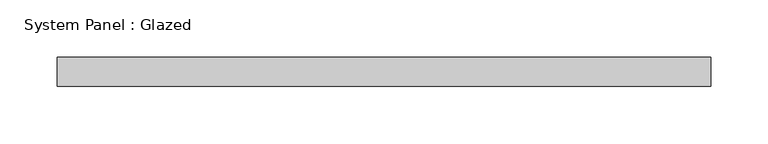
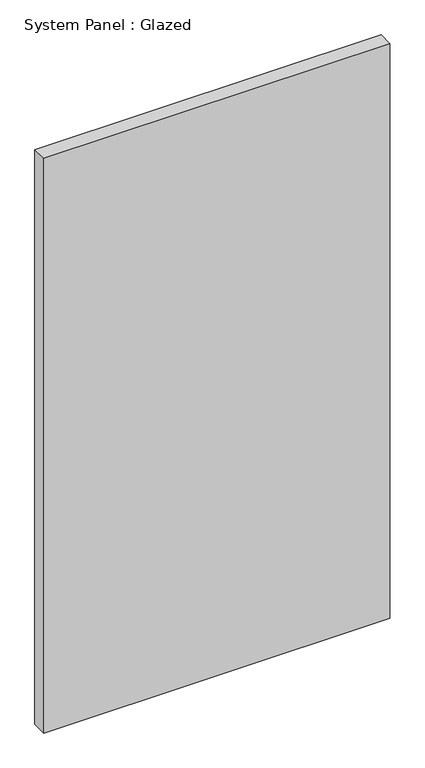
"""IFC4 building model written with IfcOpenShell, lengths in millimetres: plate geometry, System Panel : Glazed."""

from ifc_helpers import new_model, si_unit, origin, origin_with_axes, place, context, project, spatial, polyline, outline, extrude, source, transform, mapped, element, save


def system_panel_glazed_b36dd56d(model_context):
    return source(origin(), model_context, "Body", "SweptSolid", [
        extrude(outline(polyline([(285.75, 19.05), (-285.75, 19.05), (-285.75, 44.45), (285.75, 44.45), (285.75, 19.05)])), origin_with_axes(), (0.0, 0.0, 1.0), 1003.3),
    ])


if __name__ == "__main__":
    model = new_model("IFC4")
    model_context = context("Model", 3, world=origin())
    ifc_project = project(units=[si_unit("LENGTHUNIT", "METRE", prefix="MILLI")], contexts=[model_context])
    site = spatial("IfcSite", under=ifc_project)
    building = spatial("IfcBuilding", under=site)
    placement = place(None, origin())
    system_panel_glazed_shape = system_panel_glazed_b36dd56d(model_context)
    element("IfcPlate", 1, ObjectType="System Panel : Glazed", at=placement, inside=building, context=model_context, shape_type="MappedRepresentation", body=[
        mapped(system_panel_glazed_shape, transform((0.0, 0.0, 0.0), x_axis=(1.0, 0.0, 0.0), y_axis=(0.0, 1.0, 0.0), z_axis=(0.0, 0.0, 1.0))),
    ])
    save(model, "model.ifc")

# Revit data of these elements
# Type "System Panel : Glazed"
#   Construction Type Id = "GSP4R"
#   Analytic Construction = "1/8 in Pilkington single glazing"
#   Visual Light Transmittance = 0.9
#   Solar Heat Gain Coefficient = 0.86
#   Heat Transfer Coefficient (U) = 1.18115 BTU/(h·ft²·°F)
#   Define Thermal Properties by = 1
# Element 1 (IfcPlate, "System Panel : Glazed")
#   Materials on its faces: "Glass"
# Materials
#   "Glass": class "Glass", colour RGB 0 128 192, transparency 0.75, Description = "Soda Lime Glass", Cost = 0
